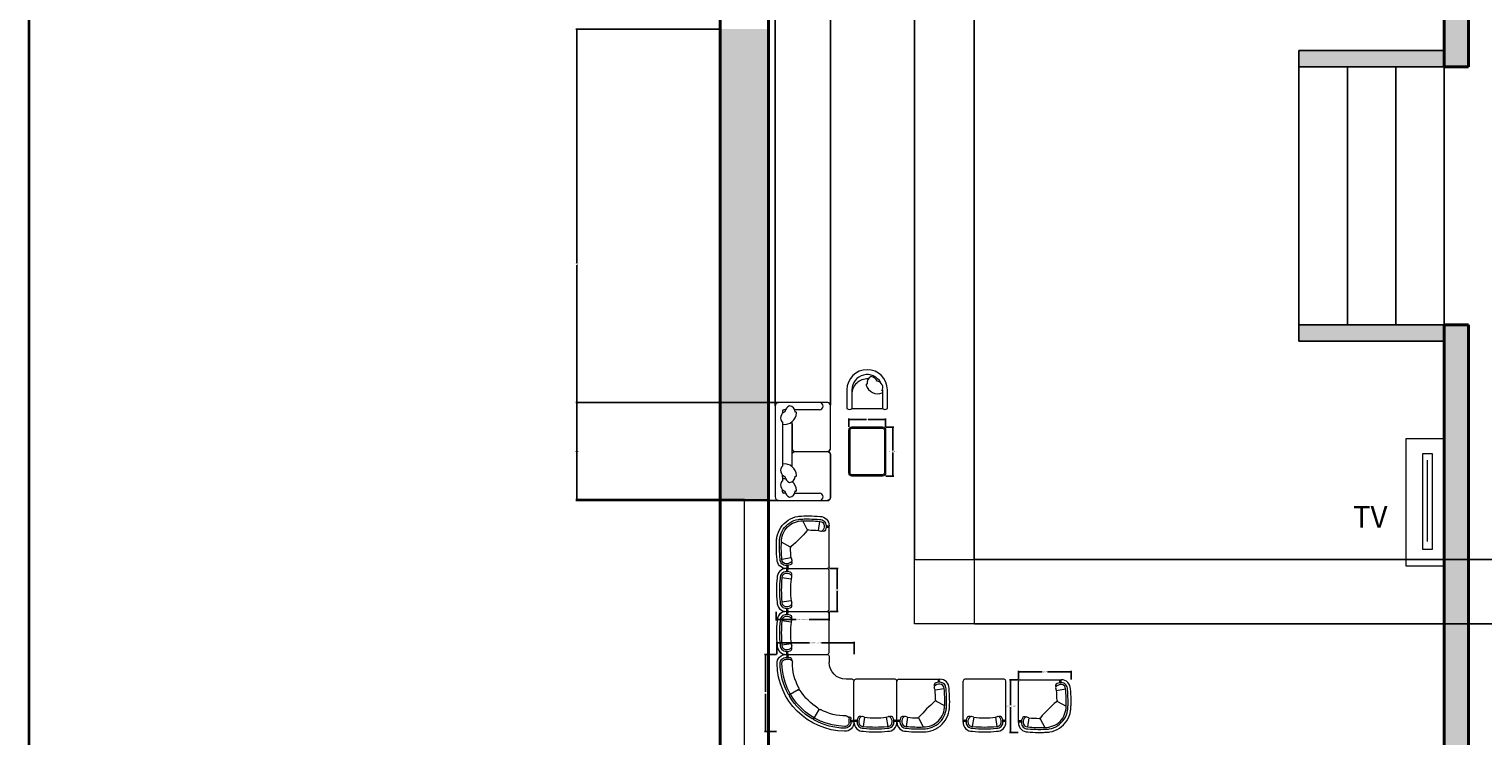
# Model space of a CAD drawing. Units: inches. Extents: x 1441 to 2460, y 1648 to 2683.
# Tile 11 of 35: x 1441 to 1711, y 1975 to 2107. Entities that reach past the tile are written whole.
import ezdxf

# ---------------------------------------------------------------- set-up
doc = ezdxf.new("R2010")
doc.units = ezdxf.units.IN
for name, color, linetype, lineweight in [('A-ANNO-DIMS', 2, 'Continuous', 18), ('A-ANNO-TEXT', 7, 'Continuous', 18), ('A-ANNO-TTLB', 7, 'Continuous', 35), ('A-EQPM', 8, 'Continuous', 18), ('A-FLOR-STRS', 7, 'Continuous', 25), ('A-FURN', 8, 'Continuous', 15), ('A-GLAZ', 4, 'Continuous', 18), ('A-WALL', 7, 'Continuous', 40)]:
    doc.layers.add(name, color=color, linetype=linetype, lineweight=lineweight)
doc.layers.add('A-WALL-PATT', color=251, linetype='Continuous', lineweight=13, true_color=0x636466)
doc.styles.get("Standard").update_dxf_attribs({"font": 'arial.ttf'})
doc.dimstyles.get("Standard").update_dxf_attribs({"dimtxt": 0.18, "dimasz": 0.18, "dimexe": 0.18, "dimexo": 0.0625, "dimgap": 0.09, "dimtad": 0, "dimtih": 1, "dimtoh": 1, "dimdec": 4, "dimzin": 0, "dimdsep": 46, "dimtxsty": 'Standard', "dimcen": 0.09, "dimadec": 0, "dimazin": 0, "dimtfac": 1, "dimtdec": 4, "dimtofl": 0, "dimtmove": 0, "dimatfit": 3, "dimfxl": 1, "dimtolj": 1, "dimtzin": 0, "dimarcsym": 0})

# ---------------------------------------------------------------- blocks, each defined once
blk = doc.blocks.new('A$C707258B2')
at = {"color": 0}
for p, q in [((0.404, 0.342), (1.074, 0.342)), ((0.404, 0.292), (0.454, 0.292)), ((0.404, 0.262), (0.454, 0.262)), ((1.104, 0.312), (1.104, 0.212)), ((1.479, -0.063), (1.379, -0.063)), ((1.509, -0.763), (1.509, -0.093)), ((0.6, -0.238), (0.47, -0.313)), ((0.929, -0.567), (0.854, -0.697)), ((1.429, -0.763), (1.429, -0.713)), ((1.459, -0.763), (1.459, -0.712))]:
    blk.add_line(p, q, dxfattribs=at)
for centre, radius, start, end in [((0.404, 0.192), 0.15, 90, 181.1754), ((0.404, 0.192), 0.1, 90, 181.1754), ((0.404, 0.192), 0.07, 90, 181.1754), ((0.378, 0.317), 0.0362, 316.3972, 43.6028), ((0.368, 0.317), 0.0662, 337.8298, 22.1702), ((0.455, 0.256), 0.0357, 345.4262, 90.5555), ((0.454, 0.212), 0.05, 360, 90), ((1.074, 0.312), 0.03, 360, 90), ((1.379, 0.212), 1.125, 181.1754, 268.8246), ((1.379, 0.212), 1.075, 181.1754, 208.6357), ((1.379, 0.212), 1.045, 181.1754, 268.8246), ((1.379, 0.212), 0.875, 180, 208.4082), ((1.379, 0.212), 0.275, 180, 270), ((0.587, -0.216), 0.025, 300, 28.4082), ((0.612, -0.259), 0.025, 31.5918, 120), ((1.479, -0.093), 0.03, 360, 90), ((0.457, -0.291), 0.025, 208.6357, 300), ((0.482, -0.334), 0.025, 120, 211.3643), ((1.379, 0.212), 1.075, 211.3643, 238.6357), ((1.379, 0.212), 0.875, 211.5918, 238.4082), ((0.832, -0.685), 0.025, 238.6357, 330), ((0.876, -0.71), 0.025, 150, 241.3643), ((0.907, -0.555), 0.025, 330, 58.4082), ((0.951, -0.58), 0.025, 61.5918, 150), ((1.379, 0.212), 0.875, 241.5918, 270), ((1.379, -0.713), 0.05, 360, 90), ((1.425, -0.709), 0.0336, 354.6301, 109.3883), ((1.379, 0.212), 1.075, 241.3643, 268.8246), ((1.359, -0.763), 0.15, 268.8246, 360), ((1.359, -0.763), 0.1, 268.8246, 360), ((1.359, -0.763), 0.07, 268.8246, 360), ((1.484, -0.799), 0.0662, 67.8298, 112.1702), ((1.484, -0.789), 0.0362, 46.3972, 133.6028)]:
    blk.add_arc(centre, radius, start, end, dxfattribs=at)
blk = doc.blocks.new('A$C1352')
at = {"color": 0}
for points in [[(0.003, 0.053), (0.003, 0.553, -0.414214), (0.053, 0.603), (0.753, 0.603, -0.414214), (0.803, 0.553), (0.803, 0.053, -0.414214), (0.753, 0.003), (0.053, 0.003, -0.414214)], [(0.023, 0.053), (0.023, 0.553, -0.414214), (0.053, 0.583), (0.753, 0.583, -0.414214), (0.783, 0.553), (0.783, 0.053, -0.414214), (0.753, 0.023), (0.053, 0.023, -0.414214)]]:
    blk.add_lwpolyline(points, format="xyb", close=True, dxfattribs=at)
blk = doc.blocks.new('part 01')
at = {"color": 0}
for p, q in [((-591, 527), (-740, 550)), ((-670, 700), (0, 700)), ((-591, 527), (-579, 561)), ((30, 30), (30, 670)), ((-591, 173), (-740, 150)), ((-670, 0), (0, 0)), ((-591, 173), (-579, 139))]:
    blk.add_line(p, q, dxfattribs=at)
for centre, radius, start, end in [((1178, 350), 2008, 174.2835, 185.7165), ((-670, 550), 150, 90, 181.1754), ((1178, 350), 1958, 174.2835, 185.7165), ((-670, 550), 100, 90, 181.1754), ((1178, 350), 1928, 174.2835, 185.7165), ((-670, 550), 70, 90, 181.1754), ((-660, 518), 133, 56.0897, 95.6132), ((-696, 675), 36.2, 316.3972, 43.6028), ((-660, 518), 103, 42.0066, 95.6132), ((-706, 675), 66.2, 337.8298, 22.1702), ((1178, 350), 1778, 174.2835, 185.7165), ((-600, 607), 25, 332.9608, 56.0897), ((-625, 620), 53.2, 321.0017, 332.9608), ((-602, 570), 25, 340, 42.0066), ((0, 670), 30, 0, 90), ((-670, 150), 150, 178.8246, 270), ((-670, 150), 100, 178.8246, 270), ((-670, 150), 70, 178.8246, 270), ((-660, 182), 133, 264.3868, 303.9103), ((-660, 182), 103, 264.3868, 317.9934), ((-696, 25), 36.2, 316.3972, 43.6028), ((-706, 25), 66.2, 337.8298, 22.1702), ((-600, 93), 25, 303.9103, 27.0392), ((-602, 130), 25, 317.9934, 20), ((-625, 80), 53.2, 27.0392, 38.9983), ((0, 30), 30, 270, 0)]:
    blk.add_arc(centre, radius, start, end, dxfattribs=at)
blk = doc.blocks.new('part02')
at = {"color": 0}
for p, q in [((0, -670), (0, 0)), ((30, 30), (700, 30)), ((621, -143), (609, -109)), ((621, -143), (770, -120)), ((640, -326), (778, -399)), ((173, -591), (139, -579)), ((173, -591), (150, -740)), ((356, -610), (429, -748))]:
    blk.add_line(p, q, dxfattribs=at)
for centre, radius, start, end in [((30, 0), 30, 90, 180), ((726, 5), 56.2, 153.6122, 206.6666), ((726, 5), 36.2, 136.3972, 223.6028), ((700, -120), 150, 0, 90), ((630, -63), 25, 123.9103, 207.0392), ((655, -50), 53.2, 207.0392, 218.9983), ((632, -100), 25, 137.9934, 200), ((690, -152), 103, 84.3868, 137.9934), ((689, -151), 132, 85.4378, 123.9887), ((-1148, -320), 1778, 0.3836, 5.7165), ((700, -121), 101, 357.5006, 89.858), ((700, -120), 70, 0, 90), ((-1228, -320), 2008, 357.7349, 5.7032), ((-1148, -320), 1958, 355.8657, 5.7165), ((-1148, -320), 2008, 355.818, 5.7165), ((2220, -2190), 2454, 130.6961, 139.3039), ((439, -409), 419, 268.2181, 1.7819), ((439, -409), 369, 268.2181, 1.7819), ((439, -409), 339, 268.2181, 1.7819), ((632, -344), 20, 62, 130.6961), ((650, -308), 20, 180.3836, 242), ((25, -696), 56.2, 63.3334, 116.3878), ((25, -696), 36.2, 46.3972, 133.6028), ((150, -670), 150, 180, 271.1754), ((182, -660), 133, 146.0897, 185.6132), ((150, -670), 100, 180, 271.1754), ((93, -600), 25, 62.9608, 146.0897), ((182, -660), 103, 132.0066, 185.6132), ((150, -670), 70, 180, 270), ((80, -625), 53.2, 51.0017, 62.9608), ((130, -602), 25, 70, 132.0066), ((350, 1178), 1778, 264.2835, 269.6164), ((338, -620), 20, 28, 89.6164), ((374, -602), 20, 139.3039, 208), ((350, 1258), 2008, 264.2968, 272.2651), ((350, 1178), 2008, 264.2835, 274.182), ((350, 1178), 1958, 264.2835, 274.1343)]:
    blk.add_arc(centre, radius, start, end, dxfattribs=at)
blk = doc.blocks.new('*D24')
at = {"layer": 'A-ANNO-DIMS', "color": 0, "lineweight": -2, "transparency": 16777216}
for p, q in [((1579.29, 1998.38), (1579.29, 1996.79)), ((1589.12, 1998.38), (1589.12, 1996.79)), ((1579.47, 1996.97), (1582.99, 1996.97)), ((1588.94, 1996.97), (1585.43, 1996.97))]:
    blk.add_line(p, q, dxfattribs=at)
at = {"layer": 'A-ANNO-DIMS', "color": 0, "transparency": 16777216}
for points in [[(1579.47, 1997), (1579.47, 1996.94), (1579.29, 1996.97)], [(1588.94, 1997), (1588.94, 1996.94), (1589.12, 1996.97)]]:
    blk.add_solid(points, dxfattribs=at)
at = {"layer": 'Defpoints', "color": 0, "transparency": 16777216}
for p in [(1579.29, 1998.44), (1589.12, 1998.44), (1589.12, 1996.97)]:
    blk.add_point(p, dxfattribs=at)
at = {"layer": 'A-ANNO-DIMS', "color": 0, "transparency": 16777216, "insert": (1584.21, 1996.97), "char_height": 0.18, "attachment_point": 5}
blk.add_mtext('\\A1;SEAT UNIT 10 TYP.', dxfattribs=at)
blk = doc.blocks.new('*D25')
at = {"layer": 'A-ANNO-DIMS', "color": 0, "lineweight": -2, "transparency": 16777216}
for p, q in [((1589.19, 2006.42), (1590.78, 2006.42)), ((1590.6, 2006.24), (1590.6, 2002.61)), ((1590.6, 1998.62), (1590.6, 2002.25)), ((1589.19, 1998.44), (1590.78, 1998.44))]:
    blk.add_line(p, q, dxfattribs=at)
at = {"layer": 'A-ANNO-DIMS', "color": 0, "transparency": 16777216}
for points in [[(1590.57, 2006.24), (1590.63, 2006.24), (1590.6, 2006.42)], [(1590.57, 1998.62), (1590.63, 1998.62), (1590.6, 1998.44)]]:
    blk.add_solid(points, dxfattribs=at)
at = {"layer": 'Defpoints', "color": 0, "transparency": 16777216}
for p in [(1589.12, 2006.42), (1590.6, 2006.42), (1589.12, 1998.44)]:
    blk.add_point(p, dxfattribs=at)
at = {"layer": 'A-ANNO-DIMS', "color": 0, "transparency": 16777216, "insert": (1590.6, 2002.43), "char_height": 0.18, "attachment_point": 5}
blk.add_mtext('\\A1;8 TYP.', dxfattribs=at)
blk = doc.blocks.new('*D26')
at = {"layer": 'A-ANNO-DIMS', "color": 0, "lineweight": -2, "transparency": 16777216}
for p, q in [((1624.21, 1985.76), (1622.62, 1985.76)), ((1622.8, 1985.58), (1622.8, 1981.02)), ((1622.8, 1976.11), (1622.8, 1980.66)), ((1624.21, 1975.93), (1622.62, 1975.93))]:
    blk.add_line(p, q, dxfattribs=at)
at = {"layer": 'A-ANNO-DIMS', "color": 0, "transparency": 16777216}
for points in [[(1622.77, 1985.58), (1622.83, 1985.58), (1622.8, 1985.76)], [(1622.77, 1976.11), (1622.83, 1976.11), (1622.8, 1975.93)]]:
    blk.add_solid(points, dxfattribs=at)
at = {"layer": 'Defpoints', "color": 0, "transparency": 16777216}
for p in [(1622.8, 1985.76), (1624.27, 1985.76), (1624.27, 1975.93)]:
    blk.add_point(p, dxfattribs=at)
at = {"layer": 'A-ANNO-DIMS', "color": 0, "transparency": 16777216, "insert": (1622.8, 1980.84), "char_height": 0.18, "attachment_point": 5}
blk.add_mtext('\\A1;END UNIT 10 TYP.', dxfattribs=at)
blk = doc.blocks.new('*D27')
at = {"layer": 'A-ANNO-DIMS', "color": 0, "lineweight": -2, "transparency": 16777216}
for p, q in [((1624.27, 1985.82), (1624.27, 1987.41)), ((1624.45, 1987.23), (1628.67, 1987.23)), ((1633.92, 1987.23), (1629.71, 1987.23)), ((1634.1, 1985.82), (1634.1, 1987.41))]:
    blk.add_line(p, q, dxfattribs=at)
at = {"layer": 'A-ANNO-DIMS', "color": 0, "transparency": 16777216}
for points in [[(1624.45, 1987.26), (1624.45, 1987.2), (1624.27, 1987.23)], [(1633.92, 1987.26), (1633.92, 1987.2), (1634.1, 1987.23)]]:
    blk.add_solid(points, dxfattribs=at)
at = {"layer": 'Defpoints', "color": 0, "transparency": 16777216}
for p in [(1624.27, 1985.76), (1634.1, 1987.23), (1634.1, 1985.76)]:
    blk.add_point(p, dxfattribs=at)
at = {"layer": 'A-ANNO-DIMS', "color": 0, "transparency": 16777216, "insert": (1629.19, 1987.23), "char_height": 0.18, "attachment_point": 5}
blk.add_mtext('\\A1;10 TYP.', dxfattribs=at)
blk = doc.blocks.new('*D28')
at = {"layer": 'A-ANNO-DIMS', "color": 0, "lineweight": -2, "transparency": 16777216}
for p, q in [((1579.43, 1990.53), (1579.43, 1992.79)), ((1579.61, 1992.61), (1585.46, 1992.61)), ((1593.56, 1992.61), (1587.71, 1992.61)), ((1593.74, 1990.53), (1593.74, 1992.79))]:
    blk.add_line(p, q, dxfattribs=at)
at = {"layer": 'A-ANNO-DIMS', "color": 0, "transparency": 16777216}
for points in [[(1579.61, 1992.64), (1579.61, 1992.58), (1579.43, 1992.61)], [(1593.56, 1992.64), (1593.56, 1992.58), (1593.74, 1992.61)]]:
    blk.add_solid(points, dxfattribs=at)
at = {"layer": 'Defpoints', "color": 0, "transparency": 16777216}
for p in [(1579.43, 1990.47), (1593.74, 1992.61), (1593.74, 1990.47)]:
    blk.add_point(p, dxfattribs=at)
at = {"layer": 'A-ANNO-DIMS', "color": 0, "transparency": 16777216, "insert": (1586.59, 1992.61), "char_height": 0.18, "attachment_point": 5}
blk.add_mtext('\\A1;CORNER UNIT 14', dxfattribs=at)
blk = doc.blocks.new('*D29')
at = {"layer": 'A-ANNO-DIMS', "color": 0, "lineweight": -2, "transparency": 16777216}
for p, q in [((1579.37, 1990.47), (1577.11, 1990.47)), ((1577.29, 1990.29), (1577.29, 1983.5)), ((1577.29, 1976.34), (1577.29, 1983.13)), ((1579.37, 1976.16), (1577.11, 1976.16))]:
    blk.add_line(p, q, dxfattribs=at)
at = {"layer": 'A-ANNO-DIMS', "color": 0, "transparency": 16777216}
for points in [[(1577.26, 1990.29), (1577.32, 1990.29), (1577.29, 1990.47)], [(1577.26, 1976.34), (1577.32, 1976.34), (1577.29, 1976.16)]]:
    blk.add_solid(points, dxfattribs=at)
at = {"layer": 'Defpoints', "color": 0, "transparency": 16777216}
for p in [(1577.29, 1990.47), (1579.43, 1990.47), (1579.43, 1976.16)]:
    blk.add_point(p, dxfattribs=at)
at = {"layer": 'A-ANNO-DIMS', "color": 0, "transparency": 16777216, "insert": (1577.29, 1983.32), "char_height": 0.18, "attachment_point": 5}
blk.add_mtext('\\A1;14', dxfattribs=at)
blk = doc.blocks.new('*D30')
at = {"layer": 'A-ANNO-DIMS', "color": 0, "lineweight": -2, "transparency": 16777216}
for p, q in [((1599.67, 2032.73), (1601.15, 2032.73)), ((1600.97, 2032.55), (1600.97, 2028.36)), ((1600.97, 2023.8), (1600.97, 2027.99)), ((1599.67, 2023.62), (1601.15, 2023.62))]:
    blk.add_line(p, q, dxfattribs=at)
at = {"layer": 'A-ANNO-DIMS', "color": 0, "transparency": 16777216}
for points in [[(1600.94, 2032.55), (1601, 2032.55), (1600.97, 2032.73)], [(1600.94, 2023.8), (1601, 2023.8), (1600.97, 2023.62)]]:
    blk.add_solid(points, dxfattribs=at)
at = {"layer": 'Defpoints', "color": 0, "transparency": 16777216}
for p in [(1599.61, 2032.73), (1600.97, 2032.73), (1599.61, 2023.62)]:
    blk.add_point(p, dxfattribs=at)
at = {"layer": 'A-ANNO-DIMS', "color": 0, "transparency": 16777216, "insert": (1600.97, 2028.17), "char_height": 0.18, "attachment_point": 5}
blk.add_mtext('\\A1;OTTOMAN 9', dxfattribs=at)
blk = doc.blocks.new('*D31')
at = {"layer": 'A-ANNO-DIMS', "color": 0, "lineweight": -2, "transparency": 16777216}
for p, q in [((1592.77, 2032.79), (1592.77, 2034.28)), ((1592.95, 2034.1), (1596.04, 2034.1)), ((1599.43, 2034.1), (1596.34, 2034.1)), ((1599.61, 2032.79), (1599.61, 2034.28))]:
    blk.add_line(p, q, dxfattribs=at)
at = {"layer": 'A-ANNO-DIMS', "color": 0, "transparency": 16777216}
for points in [[(1592.95, 2034.13), (1592.95, 2034.07), (1592.77, 2034.1)], [(1599.43, 2034.13), (1599.43, 2034.07), (1599.61, 2034.1)]]:
    blk.add_solid(points, dxfattribs=at)
at = {"layer": 'Defpoints', "color": 0, "transparency": 16777216}
for p in [(1592.77, 2034.1), (1592.77, 2032.73), (1599.61, 2032.73)]:
    blk.add_point(p, dxfattribs=at)
at = {"layer": 'A-ANNO-DIMS', "color": 0, "transparency": 16777216, "insert": (1596.19, 2034.1), "char_height": 0.18, "attachment_point": 5}
blk.add_mtext('\\A1;7', dxfattribs=at)
blk = doc.blocks.new('*D77')
at = {"layer": 'A-ANNO-DIMS', "color": 0, "lineweight": -2, "transparency": 16777216}
for p, q in [((1568.82, 2106.69), (1542.06, 2106.69)), ((1542.24, 2106.51), (1542.24, 2063.15)), ((1542.24, 2019.42), (1542.24, 2062.78)), ((1568.82, 2019.24), (1542.06, 2019.24))]:
    blk.add_line(p, q, dxfattribs=at)
at = {"layer": 'A-ANNO-DIMS', "color": 0, "transparency": 16777216}
for points in [[(1542.21, 2106.51), (1542.27, 2106.51), (1542.24, 2106.69)], [(1542.21, 2019.42), (1542.27, 2019.42), (1542.24, 2019.24)]]:
    blk.add_solid(points, dxfattribs=at)
at = {"layer": 'Defpoints', "color": 0, "transparency": 16777216}
for p in [(1542.24, 2106.69), (1568.89, 2106.69), (1568.89, 2019.24)]:
    blk.add_point(p, dxfattribs=at)
at = {"layer": 'A-ANNO-DIMS', "color": 0, "transparency": 16777216, "insert": (1542.24, 2062.97), "char_height": 0.18, "attachment_point": 5}
blk.add_mtext('\\A1;87.45', dxfattribs=at)
blk = doc.blocks.new('*D124')
at = {"layer": 'A-ANNO-DIMS', "color": 0, "lineweight": -2, "transparency": 16777216}
for p, q in [((1604.98, 2008.16), (1604.98, 2325.53)), ((1605.16, 2325.35), (1610.06, 2325.35)), ((1615.87, 2325.35), (1610.97, 2325.35)), ((1616.05, 2008.16), (1616.05, 2325.53))]:
    blk.add_line(p, q, dxfattribs=at)
at = {"layer": 'A-ANNO-DIMS', "color": 0, "transparency": 16777216}
for points in [[(1605.16, 2325.38), (1605.16, 2325.32), (1604.98, 2325.35)], [(1615.87, 2325.38), (1615.87, 2325.32), (1616.05, 2325.35)]]:
    blk.add_solid(points, dxfattribs=at)
at = {"layer": 'Defpoints', "color": 0, "transparency": 16777216}
for p in [(1616.05, 2325.35), (1604.98, 2008.09), (1616.05, 2008.09)]:
    blk.add_point(p, dxfattribs=at)
at = {"layer": 'A-ANNO-DIMS', "color": 0, "transparency": 16777216, "insert": (1610.51, 2325.35), "char_height": 0.18, "attachment_point": 5}
blk.add_mtext('\\A1;11.075', dxfattribs=at)
blk = doc.blocks.new('*D125')
at = {"layer": 'A-ANNO-DIMS', "color": 0, "lineweight": -2, "transparency": 16777216}
for p, q in [((1616.11, 2008.09), (1916.22, 2008.09)), ((1916.04, 2007.91), (1916.04, 2002.31)), ((1916.04, 1996.35), (1916.04, 2001.95)), ((1616.11, 1996.17), (1916.22, 1996.17))]:
    blk.add_line(p, q, dxfattribs=at)
at = {"layer": 'A-ANNO-DIMS', "color": 0, "transparency": 16777216}
for points in [[(1916.01, 2007.91), (1916.07, 2007.91), (1916.04, 2008.09)], [(1916.01, 1996.35), (1916.07, 1996.35), (1916.04, 1996.17)]]:
    blk.add_solid(points, dxfattribs=at)
at = {"layer": 'Defpoints', "color": 0, "transparency": 16777216}
for p in [(1616.05, 2008.09), (1916.04, 2008.09), (1616.05, 1996.17)]:
    blk.add_point(p, dxfattribs=at)
at = {"layer": 'A-ANNO-DIMS', "color": 0, "transparency": 16777216, "insert": (1916.04, 2002.13), "char_height": 0.18, "attachment_point": 5}
blk.add_mtext('\\A1;11.922', dxfattribs=at)
blk = doc.blocks.new('*D126')
at = {"layer": 'A-ANNO-DIMS', "color": 0, "lineweight": -2, "transparency": 16777216}
for p, q in [((1579.1, 2036.67), (1579.1, 2325.53)), ((1579.28, 2325.35), (1583.77, 2325.35)), ((1589.17, 2325.35), (1584.68, 2325.35)), ((1589.35, 2036.78), (1589.35, 2325.53))]:
    blk.add_line(p, q, dxfattribs=at)
at = {"layer": 'A-ANNO-DIMS', "color": 0, "transparency": 16777216}
for points in [[(1579.28, 2325.38), (1579.28, 2325.32), (1579.1, 2325.35)], [(1589.17, 2325.38), (1589.17, 2325.32), (1589.35, 2325.35)]]:
    blk.add_solid(points, dxfattribs=at)
at = {"layer": 'Defpoints', "color": 0, "transparency": 16777216}
for p in [(1589.35, 2325.35), (1579.1, 2036.6), (1589.35, 2036.72)]:
    blk.add_point(p, dxfattribs=at)
at = {"layer": 'A-ANNO-DIMS', "color": 0, "transparency": 16777216, "insert": (1584.23, 2325.35), "char_height": 0.18, "attachment_point": 5}
blk.add_mtext('\\A1;10.253', dxfattribs=at)
blk = doc.blocks.new('*D127')
at = {"layer": 'A-ANNO-DIMS', "color": 0, "lineweight": -2, "transparency": 16777216}
for p, q in [((1579.72, 2037.29), (1542.06, 2037.29)), ((1542.24, 2037.11), (1542.24, 2028.36)), ((1542.24, 2019.24), (1542.24, 2027.99)), ((1579.72, 2019.06), (1542.06, 2019.06))]:
    blk.add_line(p, q, dxfattribs=at)
at = {"layer": 'A-ANNO-DIMS', "color": 0, "transparency": 16777216}
for points in [[(1542.21, 2037.11), (1542.27, 2037.11), (1542.24, 2037.29)], [(1542.21, 2019.24), (1542.27, 2019.24), (1542.24, 2019.06)]]:
    blk.add_solid(points, dxfattribs=at)
at = {"layer": 'Defpoints', "color": 0, "transparency": 16777216}
for p in [(1542.24, 2037.29), (1579.78, 2037.29), (1579.78, 2019.06)]:
    blk.add_point(p, dxfattribs=at)
at = {"layer": 'A-ANNO-DIMS', "color": 0, "transparency": 16777216, "insert": (1542.24, 2028.17), "char_height": 0.18, "attachment_point": 5}
blk.add_mtext('\\A1;18.228', dxfattribs=at)

msp = doc.modelspace()

# ---------------------------------------------------------------- hatches: boundary and pattern name
at = {"layer": 'A-WALL-PATT'}
h = msp.add_hatch(color=256, dxfattribs=at)
h.dxf.hatch_style = 1
h.paths.add_polyline_path([(1627.5085, 2298.6952), (1568.8859, 2298.6952), (1568.8859, 2246.9605), (1577.8859, 2246.9605), (1577.8859, 2289.6952), (1627.5085, 2289.6952), (1627.5085, 2294.1952)])
h.paths.add_polyline_path([(1675.5777, 2298.6952), (1651.5085, 2298.6952), (1651.5085, 2289.6952), (1675.5777, 2289.6952), (1675.5777, 2294.1952)])
h.paths.add_polyline_path([(1667.3859, 2289.6952), (1662.8859, 2289.6952), (1662.8859, 2233.0622), (1667.3859, 2233.0622)])
h.paths.add_polyline_path([(1715.8721, 2294.3362), (1715.8721, 2295.2788), (1715.8721, 2298.6952), (1699.5777, 2298.6952), (1699.5777, 2289.6952), (1715.8721, 2289.6952)])
h.paths.add_polyline_path([(1707.8859, 2289.6952), (1703.3859, 2289.6952), (1703.3859, 2199.6952), (1707.8859, 2199.6952)])
h.paths.add_polyline_path([(1760.3859, 2204.637), (1755.8859, 2204.637), (1755.8859, 2199.6952), (1667.3859, 2199.6952), (1667.3859, 2204.637), (1662.8859, 2204.637), (1662.8859, 2195.1952), (1760.3859, 2195.1952)])
h.paths.add_polyline_path([(1760.3859, 2289.6952), (1755.8859, 2289.6952), (1755.8859, 2233.0622), (1760.3859, 2233.0622)])
h.paths.add_polyline_path([(1889.3859, 2298.6952), (1739.8721, 2298.6952), (1739.8721, 2289.6952), (1880.3859, 2289.6952), (1880.3859, 2250.8051), (1889.3859, 2250.8051)])
h.paths.add_polyline_path([(1889.3859, 2202.8051), (1880.3859, 2202.8051), (1880.3859, 2157.6952), (1747.948, 2157.6952), (1747.948, 2153.1952), (1755.8859, 2153.1952), (1755.8859, 2058.005), (1760.3859, 2058.005), (1760.3859, 2153.1952), (1880.3859, 2153.1952), (1880.3859, 2124.108), (1889.3859, 2124.108)])
h.paths.add_polyline_path([(1889.3859, 1984.8305), (1880.3859, 1984.8305), (1880.3859, 1834.1952), (1889.3859, 1834.1952)])
h.paths.add_polyline_path([(1889.3859, 2076.108), (1880.3859, 2076.108), (1880.3859, 2008.8305), (1889.3859, 2008.8305)])
h.paths.add_polyline_path([(1880.3859, 2027.1952), (1800.8859, 2027.1952), (1800.8859, 2000.9452), (1805.3859, 2000.9452), (1805.3859, 2022.6952), (1880.3859, 2022.6952)])
h.paths.add_polyline_path([(1800.8859, 2027.1952), (1760.3859, 2027.1952), (1760.3859, 2030.7912), (1755.8859, 2030.7912), (1755.8859, 2022.6952), (1800.8859, 2022.6952)])
h.paths.add_polyline_path([(1880.3859, 1974.6952), (1805.3859, 1974.6952), (1805.3859, 1978.7973), (1800.8859, 1978.7973), (1800.8859, 1974.6952), (1794.8823, 1974.6952), (1794.8823, 1970.1952), (1800.8859, 1970.1952), (1805.3859, 1970.1952), (1880.3859, 1970.1952)])
h.paths.add_polyline_path([(1760.3859, 1974.6952), (1755.8859, 1974.6952), (1755.8859, 1925.6952), (1751.8616, 1925.6952), (1751.8616, 1921.1952), (1760.3859, 1921.1952)])
h.paths.add_polyline_path([(1760.3859, 1921.1952), (1755.8859, 1921.1952), (1755.8859, 1843.1952), (1760.3859, 1843.1952)])
h.paths.add_polyline_path([(1799.1136, 1838.6952), (1799.1136, 1843.1952), (1760.3859, 1843.1952), (1751.8944, 1843.1952), (1751.8944, 1834.1952), (1758.1615, 1834.1952), (1799.1136, 1834.1952)])
h.paths.add_polyline_path([(1880.3859, 1843.1952), (1859.1136, 1843.1952), (1859.1136, 1834.1952), (1880.3859, 1834.1952)])
h.paths.add_polyline_path([(1577.8859, 1857.7914), (1568.8859, 1857.7914), (1568.8859, 1834.1952), (1695.0034, 1834.1952), (1695.0034, 1838.6952), (1695.0034, 1843.1952), (1577.8859, 1843.1952)])
h.paths.add_polyline_path([(1577.8859, 1959.2399), (1573.3859, 1959.2399), (1568.8859, 1959.2399), (1568.8859, 1905.7914), (1577.8859, 1905.7914), (1577.8859, 1921.1952), (1703.3859, 1921.1952), (1707.8859, 1921.1952), (1715.1501, 1921.1952), (1715.1501, 1925.6952), (1707.8859, 1925.6952), (1703.3859, 1925.6952), (1577.8859, 1925.6952)])
h.paths.add_polyline_path([(1577.8859, 2106.6907), (1568.8859, 2106.6907), (1568.8859, 2019.2399), (1577.8859, 2019.2399)])
h.paths.add_polyline_path([(1707.8859, 2051.6952), (1703.3859, 2051.6952), (1703.3859, 2048.6952), (1703.3859, 1925.6952), (1707.8859, 1925.6952)])
h.paths.add_polyline_path([(1703.3859, 2051.6952), (1676.3859, 2051.6952), (1676.3859, 2048.6952), (1703.3859, 2048.6952)])
h.paths.add_polyline_path([(1703.3859, 2102.6952), (1676.3859, 2102.6952), (1676.3859, 2099.6952), (1685.3859, 2099.6952), (1703.3859, 2099.6952)])
h.paths.add_polyline_path([(1707.8859, 2153.1952), (1710.5611, 2153.1952), (1710.5611, 2157.6952), (1707.8859, 2157.6952), (1707.8859, 2195.1952), (1703.3859, 2195.1952), (1703.3859, 2099.6952), (1707.8859, 2099.6952)])
h.paths.add_polyline_path([(1577.8859, 2198.9605), (1568.8859, 2198.9605), (1568.8859, 2166.6907), (1577.8859, 2166.6907)])

# ---------------------------------------------------------------- linework, layer by layer
at = {"layer": 'A-ANNO-TTLB'}
msp.add_lwpolyline([(1440.5107, 2682.6413), (2460.193, 2682.6413), (2460.193, 1648.08), (1440.5107, 1648.08)], close=True, dxfattribs=at)
at = {"layer": 'A-EQPM'}
msp.add_line((1700.2258, 2026.5829), (1700.2258, 2011.4315), dxfattribs=at)
for points in [[(1703.3859, 2030.5438), (1696.2198, 2030.5438), (1696.2198, 2006.9212), (1703.3859, 2006.9212)], [(1701.19, 2027.7531), (1699.3611, 2027.7531), (1699.3611, 2010.0508), (1701.19, 2010.0508)]]:
    msp.add_lwpolyline(points, close=True, dxfattribs=at)
at = {"layer": 'A-FLOR-STRS'}
for p, q in [((1703.3859, 2102.6952), (1676.3859, 2102.6952)), ((1676.3859, 2048.6952), (1676.3859, 2102.6952)), ((1703.3859, 2102.6952), (1703.3859, 2099.6952)), ((1703.3859, 2099.6952), (1703.3859, 2102.6952)), ((1703.3859, 2099.6952), (1676.3859, 2099.6952)), ((1685.3859, 2099.6952), (1676.3859, 2099.6952)), ((1676.3859, 2099.6952), (1676.3859, 2048.6952)), ((1685.3859, 2051.6952), (1685.3859, 2099.6952)), ((1703.3859, 2099.6952), (1694.3859, 2099.6952)), ((1694.3859, 2099.6952), (1694.3859, 2051.6952)), ((1703.3859, 2051.6952), (1703.3859, 2099.6952)), ((1703.3859, 2051.6952), (1676.3859, 2051.6952)), ((1694.3859, 2051.6952), (1685.3859, 2051.6952)), ((1703.3859, 2048.6952), (1703.3859, 2051.6952)), ((1703.3859, 2048.6952), (1703.3859, 2051.6952)), ((1703.3859, 2048.6952), (1676.3859, 2048.6952))]:
    msp.add_line(p, q, dxfattribs=at)
at = {"layer": 'A-FURN'}
for p, q in [((1599.0326, 2039.6268), (1599.0358, 2036.1512)), ((1580.4661, 2035.6928), (1580.4661, 2035.2736)), ((1580.4661, 2033.6288), (1580.4661, 2025.454)), ((1581.0112, 2035.9207), (1580.6939, 2035.9207)), ((1587.3016, 2035.9207), (1582.7405, 2035.9207)), ((1580.4661, 2023.3899), (1580.4661, 2023.8091)), ((1580.4661, 2023.8091), (1580.4661, 2022.7188)), ((1580.4661, 2020.6547), (1580.4661, 2021.0739)), ((1581.0112, 2020.4269), (1580.6939, 2020.4269)), ((1582.7405, 2020.4269), (1587.3016, 2020.4269))]:
    msp.add_line(p, q, dxfattribs=at)
at = {"layer": 'A-FURN', "ltscale": 0.03}
msp.add_lwpolyline([(1599.0358, 2036.1512, 0.36922868), (1599.9472, 2036.152), (1599.944, 2039.6277, 1), (1592.4249, 2039.6206), (1592.4282, 2036.145, 0.36922868), (1593.3396, 2036.1458)], format="xyb", close=True, dxfattribs=at)
at = {"layer": 'A-FURN'}
for points in [[(1598.7104, 2040.9399, 0.78508665), (1593.3363, 2039.6215), (1593.3396, 2036.1458)], [(1582.2319, 2033.3322), (1582.2319, 2028.7434, 0.41421356), (1582.8015, 2028.1738), (1588.7826, 2028.1738, 0.41421356), (1589.3522, 2028.7434), (1589.3522, 2036.7181, 0.41421356), (1588.7826, 2037.2878)], [(1582.2319, 2025.3626), (1582.2319, 2027.6041, -0.41421356), (1582.8015, 2028.1738), (1588.7826, 2028.1738, -0.41421356), (1589.3522, 2027.6041), (1589.3522, 2019.6294, -0.41421356), (1588.7826, 2019.0598)]]:
    msp.add_lwpolyline(points, format="xyb", dxfattribs=at)
at = {"layer": 'A-FURN', "ltscale": 0.03}
msp.add_lwpolyline([(1588.8965, 2028.1794, 0.41421356), (1589.3522, 2028.6351), (1589.3522, 2036.8321, 0.41421356), (1588.8965, 2037.2878), (1579.7825, 2037.2878, 0.41421356), (1579.099, 2036.6042), (1579.099, 2019.7433, 0.41421356), (1579.7825, 2019.0598), (1588.8965, 2019.0598, 0.41421356), (1589.3522, 2019.5155), (1589.3522, 2027.7125, 0.41421356), (1588.8965, 2028.1682)], format="xyb", dxfattribs=at)
at = {"layer": 'A-FURN'}
msp.add_lwpolyline([(1582.2319, 2025.3626), (1582.2319, 2033.7202)], dxfattribs=at)
msp.add_lwpolyline([(1604.9763, 2008.0936), (1616.0509, 2008.0936), (1616.0509, 1996.172), (1604.9763, 1996.172)], close=True, dxfattribs=at)
for centre, radius, start, end in [((1596.1852, 2038.8193), 2.8481, 86.341978, 180.053851), ((1597.3265, 2040.9909), 1.1708, 110.530541, 193.359681), ((1596.8039, 2040.8073), 1.2849, 18.646621, 85.000073), ((1596.1326, 2040.5956), 0.1363, 66.257677, 209.376213), ((1598.1369, 2041.1261), 2.2055, 195.714314, 292.985732), ((1597.9618, 2040.0782), 1.1415, 325.859919, 87.007779), ((1596.1844, 2039.6242), 2.8481, 0.053851, 1.146369), ((1582.203, 2035.4405), 1.2849, 109.10261, 175.456062), ((1581.6514, 2035.4912), 1.1708, 0.743002, 83.572142), ((1587.3016, 2036.6042), 0.6835, 0, 90), ((1587.3016, 2036.6042), 0.6835, 270, 0), ((1581.2577, 2034.4512), 1.1415, 107.094904, 228.242764), ((1580.6939, 2035.6928), 0.2278, 90, 180), ((1580.8325, 2035.4249), 2.2055, 261.11695, 358.388369), ((1582.9057, 2035.3988), 0.1363, 344.72647, 127.845006), ((1581.2577, 2024.6315), 1.1415, 131.757236, 252.905096), ((1580.8325, 2023.6579), 2.2055, 1.611631, 98.88305), ((1581.2577, 2021.8963), 1.1415, 131.757236, 252.905096), ((1580.8325, 2020.9226), 2.2055, 84.880983, 98.88305), ((1582.203, 2023.6423), 1.2849, 184.543938, 250.89739), ((1581.6514, 2023.5915), 1.1708, 276.427858, 359.256998), ((1582.9057, 2023.684), 0.1363, 232.154994, 15.27353), ((1580.6939, 2020.6547), 0.2278, 180, 270), ((1580.6939, 2020.6547), 0.2278, 180, 270), ((1582.203, 2020.9071), 1.2849, 184.543938, 250.89739), ((1581.6514, 2020.8563), 1.1708, 276.427858, 359.256998), ((1580.8325, 2020.9226), 2.2055, 1.611631, 49.375991), ((1582.9057, 2020.9488), 0.1363, 232.154994, 15.27353), ((1587.3016, 2019.7433), 0.6835, 0, 90), ((1587.3016, 2019.7433), 0.6835, 270, 0)]:
    msp.add_arc(centre, radius, start, end, dxfattribs=at)
at = {"layer": 'A-GLAZ'}
for p, q in [((1573.3859, 2019.2399), (1568.8859, 2019.2399)), ((1568.8859, 2019.2399), (1577.8859, 2019.2399)), ((1573.3859, 1959.2399), (1573.3859, 2019.2399))]:
    msp.add_line(p, q, dxfattribs=at)
at = {"layer": 'A-WALL'}
for p, q in [((1568.8859, 2298.6952), (1568.8859, 1834.1952)), ((1577.8859, 2289.6952), (1577.8859, 1925.6952)), ((1703.3859, 2195.1952), (1703.3859, 2099.6952)), ((1707.8859, 2153.1952), (1707.8859, 2099.6952)), ((1703.3859, 2099.6952), (1707.8859, 2099.6952)), ((1703.3859, 2051.6952), (1707.8859, 2051.6952)), ((1703.3859, 2051.6952), (1703.3859, 1925.6952)), ((1707.8859, 2051.6952), (1707.8859, 1925.6952))]:
    msp.add_line(p, q, dxfattribs=at)

# ---------------------------------------------------------------- block references
at = {"layer": 'A-FURN', "ltscale": 0.03}
for name, p, xscale, yscale, zscale, rotation in [('A$C1352', (1599.6396, 2023.5862), 11.39249584401172, 11.39249584401172, 11.39249584401172, 90), ('part02', (1588.7823, 2006.4169), -0.0113924958440117, 0.0113924958440117, 0.0113924958440117, 269.9999999999968), ('A$C707258B2', (1589.8416, 1973.2768), -11.39249584401172, 11.39249584401172, 11.39249584401172, 269.9999999999968), ('part 01', (1601.7128, 1985.5117), 0.0113924958440117, 0.0113924958440117, 0.0113924958440117, 90), ('part 01', (1621.9725, 1985.5117), 0.0113924958440117, 0.0113924958440117, 0.0113924958440117, 90)]:
    msp.add_blockref(name, p, dxfattribs=dict(at, xscale=xscale, yscale=yscale, zscale=zscale, rotation=rotation))
at = {"layer": 'A-FURN', "ltscale": 0.03, "xscale": 0.0113924958440117, "yscale": 0.0113924958440117, "zscale": 0.0113924958440117}
for name, p in [('part 01', (1588.7823, 1998.4422)), ('part 01', (1588.7823, 1990.4674)), ('part02', (1601.7128, 1985.5117)), ('part02', (1624.2715, 1985.4162))]:
    msp.add_blockref(name, p, dxfattribs=at)

# ---------------------------------------------------------------- texts
at = {"layer": 'A-ANNO-TEXT', "insert": (1686.4155, 2018.0289), "char_height": 4, "attachment_point": 1}
msp.add_mtext_dynamic_manual_height_columns('TV', width=31.556375, gutter_width=12.5, heights=[0], dxfattribs=at)

# ---------------------------------------------------------------- dimensions: what is measured, and where the dimension line sits
at = {"layer": 'A-ANNO-DIMS'}
for base, p1, p2, picture, middle in [((1589.3522, 2325.3452), (1579.099, 2036.6042), (1589.3522, 2036.7181), '*D126', (1584.2256, 2325.3452)), ((1616.0509, 2325.3452), (1604.9763, 2008.0936), (1616.0509, 2008.0936), '*D124', (1610.5136, 2325.3452))]:
    dim = msp.add_linear_dim(base=base, p1=p1, p2=p2, dimstyle='Standard', override={"dimdec": 3, "dimlfac": 1, "dimrnd": 0, "dimzin": 0, "dimdsep": 46, "dimlunit": 2}, dxfattribs=at)
    dim.commit()
    dim.dimension.update_dxf_attribs({"geometry": picture, "text_midpoint": middle})
for base, p1, p2, angle, override, picture, middle in [((1542.2359, 2106.6907), (1568.8859, 2019.2399), (1568.8859, 2106.6907), 90, {"dimdec": 2, "dimlfac": 1, "dimrnd": 0, "dimzin": 0, "dimdsep": 46, "dimlunit": 2}, '*D77', (1542.2359, 2062.9653)), ((1542.2359, 2037.2878), (1579.7825, 2019.0598), (1579.7825, 2037.2878), 90, {"dimdec": 3, "dimlfac": 1, "dimrnd": 0, "dimzin": 0, "dimdsep": 46, "dimlunit": 2}, '*D127', (1542.2359, 2028.1738)), ((1592.77, 2034.0979), (1599.6055, 2032.7308), (1592.77, 2032.7308), 180, {"dimdec": 0, "dimlfac": 1, "dimrnd": 0, "dimzin": 0, "dimdsep": 46, "dimlunit": 2}, '*D31', (1596.1877, 2034.0979)), ((1916.0359, 2008.0936), (1616.0509, 1996.172), (1616.0509, 2008.0936), 90, {"dimdec": 3, "dimlfac": 1, "dimrnd": 0, "dimzin": 0, "dimdsep": 46, "dimlunit": 2}, '*D125', (1916.0359, 2002.1328)), ((1577.2881, 1990.4674), (1579.4337, 1976.1631), (1579.4337, 1990.4674), 90, {"dimdec": 0, "dimlfac": 1, "dimrnd": 0, "dimzin": 0, "dimdsep": 46, "dimlunit": 2}, '*D29', (1577.2881, 1983.3153))]:
    dim = msp.add_linear_dim(base=base, p1=p1, p2=p2, angle=angle, dimstyle='Standard', override=override, dxfattribs=at)
    dim.commit()
    dim.dimension.update_dxf_attribs({"geometry": picture, "text_midpoint": middle})
for base, p1, p2, text, picture, middle in [((1600.9726, 2032.7308), (1599.6055, 2023.6168), (1599.6055, 2032.7308), 'OTTOMAN <>', '*D30', (1600.9726, 2028.1738)), ((1590.599, 2006.4169), (1589.1241, 1998.4422), (1589.1241, 2006.4169), '<> TYP.', '*D25', (1590.599, 2002.4295)), ((1622.797, 1985.7579), (1624.2715, 1975.9277), (1624.2715, 1985.7579), 'END UNIT <> TYP.', '*D26', (1622.797, 1980.8428))]:
    dim = msp.add_linear_dim(base=base, p1=p1, p2=p2, angle=90, text=text, dimstyle='Standard', override={"dimdec": 0, "dimlfac": 1, "dimrnd": 0, "dimzin": 0, "dimdsep": 46, "dimlunit": 2}, dxfattribs=at)
    dim.commit()
    dim.dimension.update_dxf_attribs({"geometry": picture, "text_midpoint": middle})
for base, p1, p2, text, picture, middle in [((1589.1241, 1996.9672), (1579.2911, 1998.4422), (1589.1241, 1998.4422), 'SEAT UNIT <> TYP.', '*D24', (1584.2076, 1996.9672)), ((1593.7381, 1992.6131), (1579.4337, 1990.4674), (1593.7381, 1990.4674), 'CORNER UNIT <>', '*D28', (1586.5859, 1992.6131)), ((1634.1018, 1987.2325), (1624.2715, 1985.7579), (1634.1018, 1985.7579), '<> TYP.', '*D27', (1629.1867, 1987.2325))]:
    dim = msp.add_linear_dim(base=base, p1=p1, p2=p2, text=text, dimstyle='Standard', override={"dimdec": 0, "dimlfac": 1, "dimrnd": 0, "dimzin": 0, "dimdsep": 46, "dimlunit": 2}, dxfattribs=at)
    dim.commit()
    dim.dimension.update_dxf_attribs({"geometry": picture, "text_midpoint": middle})

doc.saveas('drawing.dxf')
